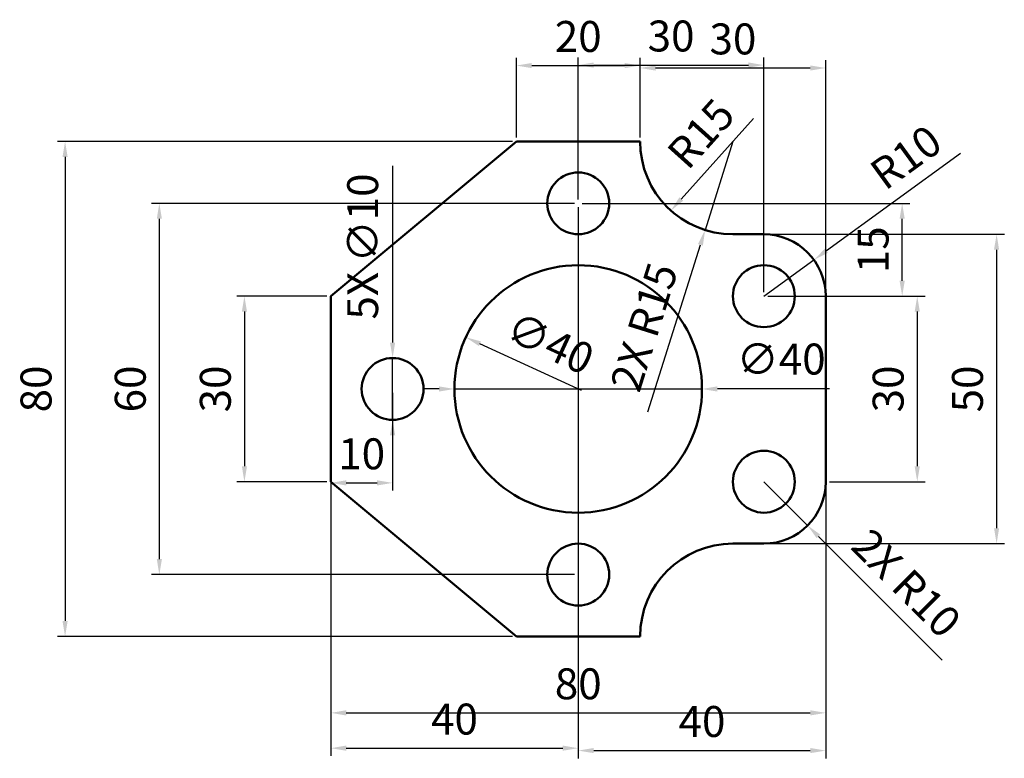
# Model space of a CAD drawing. Units: millimetres. Extents: x -90 to 69, y -60 to 60.
import ezdxf

# ---------------------------------------------------------------- set-up
doc = ezdxf.new("R2010")
doc.units = ezdxf.units.MM
doc.layers.add('M-DIMS', color=2, linetype='Continuous', lineweight=25)
doc.layers.add('M-OUTL', color=7, linetype='Continuous', lineweight=50)
doc.styles.get("Standard").update_dxf_attribs({"font": 'arial.ttf'})
doc.dimstyles.new('ISO-25', dxfattribs={"dimtxt": 5, "dimasz": 2.5, "dimexe": 1.25, "dimexo": 0.625, "dimgap": 1.5, "dimtad": 1, "dimdsep": 46, "dimtxsty": 'Standard', "dimcen": 4, "dimadec": 0, "dimazin": 0, "dimtfac": 1, "dimtmove": 0, "dimatfit": 3, "dimfxl": 1, "dimarcsym": 0})

# ---------------------------------------------------------------- blocks, each defined once
blk = doc.blocks.new('*D1')
at = {"layer": 'Defpoints', "color": 0, "transparency": 16777216}
for p in [(0, 30), (-40, -15), (0, -58.06)]:
    blk.add_point(p, dxfattribs=at)
at = {"layer": 'M-DIMS', "color": 0, "lineweight": -2, "transparency": 16777216}
for p, q in [((0, 29.38), (0, -59.31)), ((-40, -15.62), (-40, -59.31)), ((-37.5, -58.06), (-2.5, -58.06))]:
    blk.add_line(p, q, dxfattribs=at)
at = {"layer": 'M-DIMS', "color": 0, "transparency": 16777216}
for points in [[(-37.5, -57.64), (-37.5, -58.47), (-40, -58.06)], [(-2.5, -57.64), (-2.5, -58.47), (0, -58.06)]]:
    blk.add_solid(points, dxfattribs=at)
at = {"layer": 'M-DIMS', "color": 0, "transparency": 16777216, "insert": (-20, -54), "char_height": 5, "attachment_point": 5}
blk.add_mtext('40', dxfattribs=at)
blk = doc.blocks.new('*D2')
at = {"layer": 'Defpoints', "color": 0, "transparency": 16777216}
for p in [(40, -15), (0, -30), (40, -58.45)]:
    blk.add_point(p, dxfattribs=at)
at = {"layer": 'M-DIMS', "color": 0, "lineweight": -2, "transparency": 16777216}
for p, q in [((40, -15.62), (40, -59.7)), ((0, -30.62), (0, -59.7)), ((2.5, -58.45), (37.5, -58.45))]:
    blk.add_line(p, q, dxfattribs=at)
at = {"layer": 'M-DIMS', "color": 0, "transparency": 16777216}
for points in [[(2.5, -58.03), (2.5, -58.86), (0, -58.45)], [(37.5, -58.03), (37.5, -58.86), (40, -58.45)]]:
    blk.add_solid(points, dxfattribs=at)
at = {"layer": 'M-DIMS', "color": 0, "transparency": 16777216, "insert": (20, -54.39), "char_height": 5, "attachment_point": 5}
blk.add_mtext('40', dxfattribs=at)
blk = doc.blocks.new('*D3')
at = {"layer": 'Defpoints', "color": 0, "transparency": 16777216}
for p in [(-40, 15), (-53.95, -15), (-40, -15)]:
    blk.add_point(p, dxfattribs=at)
at = {"layer": 'M-DIMS', "color": 0, "lineweight": -2, "transparency": 16777216}
for p, q in [((-40.63, 15), (-55.2, 15)), ((-53.95, 12.5), (-53.95, -12.5)), ((-40.63, -15), (-55.2, -15))]:
    blk.add_line(p, q, dxfattribs=at)
at = {"layer": 'M-DIMS', "color": 0, "transparency": 16777216}
for points in [[(-54.36, 12.5), (-53.53, 12.5), (-53.95, 15)], [(-54.36, -12.5), (-53.53, -12.5), (-53.95, -15)]]:
    blk.add_solid(points, dxfattribs=at)
at = {"layer": 'M-DIMS', "color": 0, "transparency": 16777216, "insert": (-58, 0), "char_height": 5, "attachment_point": 5, "rotation": 90}
blk.add_mtext('30', dxfattribs=at)
blk = doc.blocks.new('*D4')
at = {"layer": 'Defpoints', "color": 0, "transparency": 16777216}
for p in [(0, 30), (-67.7, -30), (0, -30)]:
    blk.add_point(p, dxfattribs=at)
at = {"layer": 'M-DIMS', "color": 0, "lineweight": -2, "transparency": 16777216}
for p, q in [((-0.62, 30), (-68.95, 30)), ((-67.7, 27.5), (-67.7, -27.5)), ((-0.62, -30), (-68.95, -30))]:
    blk.add_line(p, q, dxfattribs=at)
at = {"layer": 'M-DIMS', "color": 0, "transparency": 16777216}
for points in [[(-68.11, 27.5), (-67.28, 27.5), (-67.7, 30)], [(-68.11, -27.5), (-67.28, -27.5), (-67.7, -30)]]:
    blk.add_solid(points, dxfattribs=at)
at = {"layer": 'M-DIMS', "color": 0, "transparency": 16777216, "insert": (-71.75, 0), "char_height": 5, "attachment_point": 5, "rotation": 90}
blk.add_mtext('60', dxfattribs=at)
blk = doc.blocks.new('*D5')
at = {"layer": 'Defpoints', "color": 0, "transparency": 16777216}
for p in [(-10, 40), (-82.93, -40), (-10, -40)]:
    blk.add_point(p, dxfattribs=at)
at = {"layer": 'M-DIMS', "color": 0, "lineweight": -2, "transparency": 16777216}
for p, q in [((-10.62, 40), (-84.18, 40)), ((-82.93, 37.5), (-82.93, -37.5)), ((-10.62, -40), (-84.18, -40))]:
    blk.add_line(p, q, dxfattribs=at)
at = {"layer": 'M-DIMS', "color": 0, "transparency": 16777216}
for points in [[(-83.35, 37.5), (-82.51, 37.5), (-82.93, 40)], [(-83.35, -37.5), (-82.51, -37.5), (-82.93, -40)]]:
    blk.add_solid(points, dxfattribs=at)
at = {"layer": 'M-DIMS', "color": 0, "transparency": 16777216, "insert": (-86.98, 0), "char_height": 5, "attachment_point": 5, "rotation": 90}
blk.add_mtext('80', dxfattribs=at)
blk = doc.blocks.new('*D6')
at = {"layer": 'Defpoints', "color": 0, "transparency": 16777216}
for p in [(10, 52.27), (-10, 40), (10, 40)]:
    blk.add_point(p, dxfattribs=at)
at = {"layer": 'M-DIMS', "color": 0, "lineweight": -2, "transparency": 16777216}
for p, q in [((-10, 40.62), (-10, 53.52)), ((10, 40.62), (10, 53.52)), ((-7.5, 52.27), (7.5, 52.27))]:
    blk.add_line(p, q, dxfattribs=at)
at = {"layer": 'M-DIMS', "color": 0, "transparency": 16777216}
for points in [[(-7.5, 52.69), (-7.5, 51.86), (-10, 52.27)], [(7.5, 52.69), (7.5, 51.86), (10, 52.27)]]:
    blk.add_solid(points, dxfattribs=at)
at = {"layer": 'M-DIMS', "color": 0, "transparency": 16777216, "insert": (0, 56.33), "char_height": 5, "attachment_point": 5}
blk.add_mtext('20', dxfattribs=at)
blk = doc.blocks.new('*D7')
at = {"layer": 'Defpoints', "color": 0, "transparency": 16777216}
for p in [(40, 51.88), (10, 40), (40, 15)]:
    blk.add_point(p, dxfattribs=at)
at = {"layer": 'M-DIMS', "color": 0, "lineweight": -2, "transparency": 16777216}
for p, q in [((10, 40.62), (10, 53.13)), ((40, 15.62), (40, 53.13)), ((12.5, 51.88), (37.5, 51.88))]:
    blk.add_line(p, q, dxfattribs=at)
at = {"layer": 'M-DIMS', "color": 0, "transparency": 16777216}
for points in [[(12.5, 52.29), (12.5, 51.46), (10, 51.88)], [(37.5, 52.29), (37.5, 51.46), (40, 51.88)]]:
    blk.add_solid(points, dxfattribs=at)
at = {"layer": 'M-DIMS', "color": 0, "transparency": 16777216, "insert": (25, 55.93), "char_height": 5, "attachment_point": 5}
blk.add_mtext('30', dxfattribs=at)
blk = doc.blocks.new('*D8')
at = {"layer": 'Defpoints', "color": 0, "transparency": 16777216}
for p in [(40, 15), (40, -15), (54.79, -15)]:
    blk.add_point(p, dxfattribs=at)
at = {"layer": 'M-DIMS', "color": 0, "lineweight": -2, "transparency": 16777216}
for p, q in [((40.63, 15), (56.04, 15)), ((54.79, 12.5), (54.79, -12.5)), ((40.63, -15), (56.04, -15))]:
    blk.add_line(p, q, dxfattribs=at)
at = {"layer": 'M-DIMS', "color": 0, "transparency": 16777216}
for points in [[(54.37, 12.5), (55.2, 12.5), (54.79, 15)], [(54.37, -12.5), (55.2, -12.5), (54.79, -15)]]:
    blk.add_solid(points, dxfattribs=at)
at = {"layer": 'M-DIMS', "color": 0, "transparency": 16777216, "insert": (50.73, 0), "char_height": 5, "attachment_point": 5, "rotation": 90}
blk.add_mtext('30', dxfattribs=at)
blk = doc.blocks.new('*D9')
at = {"layer": 'Defpoints', "color": 0, "transparency": 16777216}
for p in [(27.5, 25), (27.5, -25), (67.61, -25)]:
    blk.add_point(p, dxfattribs=at)
at = {"layer": 'M-DIMS', "color": 0, "lineweight": -2, "transparency": 16777216}
for p, q in [((28.13, 25), (68.86, 25)), ((67.61, 22.5), (67.61, -22.5)), ((28.13, -25), (68.86, -25))]:
    blk.add_line(p, q, dxfattribs=at)
at = {"layer": 'M-DIMS', "color": 0, "transparency": 16777216}
for points in [[(67.19, 22.5), (68.02, 22.5), (67.61, 25)], [(67.19, -22.5), (68.02, -22.5), (67.61, -25)]]:
    blk.add_solid(points, dxfattribs=at)
at = {"layer": 'M-DIMS', "color": 0, "transparency": 16777216, "insert": (63.55, 0), "char_height": 5, "attachment_point": 5, "rotation": 90}
blk.add_mtext('50', dxfattribs=at)
blk = doc.blocks.new('*D10')
at = {"layer": 'Defpoints', "color": 0, "transparency": 16777216}
for p in [(38.09, 20.87), (30, 15)]:
    blk.add_point(p, dxfattribs=at)
at = {"layer": 'M-DIMS', "color": 0, "lineweight": -2, "transparency": 16777216}
for p, q in [((61.76, 38.04), (40.12, 22.34)), ((30, 15), (38.09, 20.87))]:
    blk.add_line(p, q, dxfattribs=at)
at = {"layer": 'M-DIMS', "color": 0, "transparency": 16777216}
blk.add_solid([(39.87, 22.68), (40.36, 22), (38.09, 20.87)], dxfattribs=at)
at = {"layer": 'M-DIMS', "color": 0, "transparency": 16777216, "insert": (53.33, 36.94), "char_height": 5, "attachment_point": 5, "rotation": 35.9647}
blk.add_mtext('R10', dxfattribs=at)
blk = doc.blocks.new('*D11')
at = {"layer": 'Defpoints', "color": 0, "transparency": 16777216}
for p in [(25, 40), (14.98, 28.83)]:
    blk.add_point(p, dxfattribs=at)
at = {"layer": 'M-DIMS', "color": 0, "lineweight": -2, "transparency": 16777216}
blk.add_line((28.33, 43.71), (16.65, 30.7), dxfattribs=at)
at = {"layer": 'M-DIMS', "color": 0, "transparency": 16777216}
blk.add_solid([(16.34, 30.97), (16.96, 30.42), (14.98, 28.83)], dxfattribs=at)
at = {"layer": 'M-DIMS', "color": 0, "transparency": 16777216, "insert": (20.31, 40.84), "char_height": 5, "attachment_point": 5, "rotation": 48.1039}
blk.add_mtext('R15', dxfattribs=at)
blk = doc.blocks.new('*D12')
at = {"layer": 'Defpoints', "color": 0, "transparency": 16777216}
for p in [(-40, 0), (-30, 0), (-30, -15.18)]:
    blk.add_point(p, dxfattribs=at)
at = {"layer": 'M-DIMS', "color": 0, "lineweight": -2, "transparency": 16777216}
for p, q in [((-40, -0.62), (-40, -16.43)), ((-30, -0.62), (-30, -16.43)), ((-37.5, -15.18), (-32.5, -15.18))]:
    blk.add_line(p, q, dxfattribs=at)
at = {"layer": 'M-DIMS', "color": 0, "transparency": 16777216}
for points in [[(-37.5, -14.76), (-37.5, -15.6), (-40, -15.18)], [(-32.5, -14.76), (-32.5, -15.6), (-30, -15.18)]]:
    blk.add_solid(points, dxfattribs=at)
at = {"layer": 'M-DIMS', "color": 0, "transparency": 16777216, "insert": (-35, -11.13), "char_height": 5, "attachment_point": 5}
blk.add_mtext('10', dxfattribs=at)
blk = doc.blocks.new('*D13')
at = {"layer": 'Defpoints', "color": 0, "transparency": 16777216}
for p in [(-18.17, 8.36), (18.17, -8.36)]:
    blk.add_point(p, dxfattribs=at)
at = {"layer": 'M-DIMS', "color": 0, "lineweight": -2, "transparency": 16777216}
blk.add_line((0.53, -0.24), (-15.9, 7.31), dxfattribs=at)
at = {"layer": 'M-DIMS', "color": 0, "transparency": 16777216}
blk.add_solid([(-15.72, 7.69), (-16.07, 6.94), (-18.17, 8.36)], dxfattribs=at)
at = {"layer": 'M-DIMS', "color": 0, "transparency": 16777216, "insert": (-4.8, 6.82), "char_height": 5, "attachment_point": 5, "rotation": 335.2959}
blk.add_mtext('∅40', dxfattribs=at)
blk = doc.blocks.new('HOLE-D10')
blk.add_circle((5, 5), 5)
blk = doc.blocks.new('*D15')
at = {"layer": 'Defpoints', "color": 0, "transparency": 16777216}
for p in [(-40, -15), (40, -15), (40, -52.35)]:
    blk.add_point(p, dxfattribs=at)
at = {"layer": 'M-DIMS', "color": 0, "lineweight": -2, "transparency": 16777216}
for p, q in [((-40, -15.62), (-40, -53.6)), ((40, -15.62), (40, -53.6)), ((-37.5, -52.35), (37.5, -52.35))]:
    blk.add_line(p, q, dxfattribs=at)
at = {"layer": 'M-DIMS', "color": 0, "transparency": 16777216}
for points in [[(-37.5, -51.93), (-37.5, -52.77), (-40, -52.35)], [(37.5, -51.93), (37.5, -52.77), (40, -52.35)]]:
    blk.add_solid(points, dxfattribs=at)
at = {"layer": 'M-DIMS', "color": 0, "transparency": 16777216, "insert": (0, -48.3), "char_height": 5, "attachment_point": 5}
blk.add_mtext('80', dxfattribs=at)
blk = doc.blocks.new('*D16')
at = {"layer": 'Defpoints', "color": 0, "transparency": 16777216}
for p in [(30, 52.35), (0, 30), (30, 15)]:
    blk.add_point(p, dxfattribs=at)
at = {"layer": 'M-DIMS', "color": 0, "lineweight": -2, "transparency": 16777216}
for p, q in [((0, 30.62), (0, 53.6)), ((30, 15.62), (30, 53.6)), ((2.5, 52.35), (27.5, 52.35))]:
    blk.add_line(p, q, dxfattribs=at)
at = {"layer": 'M-DIMS', "color": 0, "transparency": 16777216}
for points in [[(2.5, 52.77), (2.5, 51.93), (0, 52.35)], [(27.5, 52.77), (27.5, 51.93), (30, 52.35)]]:
    blk.add_solid(points, dxfattribs=at)
at = {"layer": 'M-DIMS', "color": 0, "transparency": 16777216, "insert": (15, 56.4), "char_height": 5, "attachment_point": 5}
blk.add_mtext('30', dxfattribs=at)
blk = doc.blocks.new('*D17')
at = {"layer": 'Defpoints', "color": 0, "transparency": 16777216}
for p in [(0, 30), (52.35, 30), (30, 15)]:
    blk.add_point(p, dxfattribs=at)
at = {"layer": 'M-DIMS', "color": 0, "lineweight": -2, "transparency": 16777216}
for p, q in [((0.63, 30), (53.6, 30)), ((52.35, 17.5), (52.35, 27.5)), ((30.63, 15), (53.6, 15))]:
    blk.add_line(p, q, dxfattribs=at)
at = {"layer": 'M-DIMS', "color": 0, "transparency": 16777216}
for points in [[(51.93, 27.5), (52.77, 27.5), (52.35, 30)], [(51.93, 17.5), (52.77, 17.5), (52.35, 15)]]:
    blk.add_solid(points, dxfattribs=at)
at = {"layer": 'M-DIMS', "color": 0, "transparency": 16777216, "insert": (48.3, 22.5), "char_height": 5, "attachment_point": 5, "rotation": 90}
blk.add_mtext('15', dxfattribs=at)
blk = doc.blocks.new('*D18')
at = {"layer": 'Defpoints', "color": 0, "transparency": 16777216}
for p in [(-20, 0), (20, 0)]:
    blk.add_point(p, dxfattribs=at)
at = {"layer": 'M-DIMS', "color": 0, "lineweight": -2, "transparency": 16777216}
for p, q in [((-22.5, 0), (-25, 0)), ((-20, 0), (20, 0)), ((40.59, 0), (22.5, 0))]:
    blk.add_line(p, q, dxfattribs=at)
at = {"layer": 'M-DIMS', "color": 0, "transparency": 16777216}
for points in [[(-22.5, 0.42), (-22.5, -0.42), (-20, 0)], [(22.5, 0.42), (22.5, -0.42), (20, 0)]]:
    blk.add_solid(points, dxfattribs=at)
at = {"layer": 'M-DIMS', "color": 0, "transparency": 16777216, "insert": (32.79, 4.19), "char_height": 5, "attachment_point": 5}
blk.add_mtext('∅40', dxfattribs=at)
blk = doc.blocks.new('*D19')
at = {"layer": 'Defpoints', "color": 0, "transparency": 16777216}
for p in [(-30, 5), (-30, -5)]:
    blk.add_point(p, dxfattribs=at)
at = {"layer": 'M-DIMS', "color": 0, "lineweight": -2, "transparency": 16777216}
for p, q in [((-30, 36.06), (-30, 7.5)), ((-30, -5), (-30, 5)), ((-30, -7.5), (-30, -10))]:
    blk.add_line(p, q, dxfattribs=at)
at = {"layer": 'M-DIMS', "color": 0, "transparency": 16777216}
for points in [[(-30.42, 7.5), (-29.58, 7.5), (-30, 5)], [(-30.42, -7.5), (-29.58, -7.5), (-30, -5)]]:
    blk.add_solid(points, dxfattribs=at)
at = {"layer": 'M-DIMS', "color": 0, "transparency": 16777216, "insert": (-34.19, 23.03), "char_height": 5, "attachment_point": 5, "rotation": 90}
blk.add_mtext('5X ∅10', dxfattribs=at)
blk = doc.blocks.new('*D20')
at = {"layer": 'Defpoints', "color": 0, "transparency": 16777216}
for p in [(25, 40), (20.5, 25.69)]:
    blk.add_point(p, dxfattribs=at)
at = {"layer": 'M-DIMS', "color": 0, "lineweight": -2, "transparency": 16777216}
for p, q in [((25, 40), (20.5, 25.69)), ((11.26, -3.7), (19.75, 23.31))]:
    blk.add_line(p, q, dxfattribs=at)
at = {"layer": 'M-DIMS', "color": 0, "transparency": 16777216}
blk.add_solid([(19.35, 23.43), (20.15, 23.18), (20.5, 25.69)], dxfattribs=at)
at = {"layer": 'M-DIMS', "color": 0, "transparency": 16777216, "insert": (11.26, 9.82), "char_height": 5, "attachment_point": 5, "rotation": 72.5434}
blk.add_mtext('2X R15', dxfattribs=at)
blk = doc.blocks.new('*D21')
at = {"layer": 'Defpoints', "color": 0, "transparency": 16777216}
for p in [(30, -15), (37.07, -22.07)]:
    blk.add_point(p, dxfattribs=at)
at = {"layer": 'M-DIMS', "color": 0, "lineweight": -2, "transparency": 16777216}
for p, q in [((30, -15), (37.07, -22.07)), ((58.82, -43.82), (38.84, -23.84))]:
    blk.add_line(p, q, dxfattribs=at)
at = {"layer": 'M-DIMS', "color": 0, "transparency": 16777216}
blk.add_solid([(39.13, -23.54), (38.54, -24.13), (37.07, -22.07)], dxfattribs=at)
at = {"layer": 'M-DIMS', "color": 0, "transparency": 16777216, "insert": (52.58, -31.85), "char_height": 5, "attachment_point": 5, "rotation": 315}
blk.add_mtext('2X R10', dxfattribs=at)

msp = doc.modelspace()

# ---------------------------------------------------------------- linework, layer by layer
at = {"layer": 'M-OUTL'}
for p, q in [((-10, 40), (-40, 15)), ((0, 40), (-10, 40)), ((0, 40), (10, 40)), ((10, 40), (10, 40)), ((25, 25), (30, 25)), ((-40, 0), (-40, 15)), ((40, 15), (40, 0)), ((-40, 0), (-40, -15)), ((40, -15), (40, 0)), ((-10, -40), (-40, -15)), ((25, -25), (30, -25)), ((0, -40), (-10, -40)), ((0, -40), (10, -40)), ((10, -40), (10, -40))]:
    msp.add_line(p, q, dxfattribs=at)
msp.add_circle((0, 0), 20, dxfattribs=at)
for centre, radius, start, end in [((25, 40), 15, 180, 270), ((30, 15), 10, 0, 90), ((30, -15), 10, 270, 0), ((25, -40), 15, 90, 180)]:
    msp.add_arc(centre, radius, start, end, dxfattribs=at)

# ---------------------------------------------------------------- block references
for p in [(-5, 25), (25, 10), (-35, -5), (25, -20), (-5, -35)]:
    msp.add_blockref('HOLE-D10', p, dxfattribs=at)

# ---------------------------------------------------------------- dimensions: what is measured, and where the dimension line sits
at = {"layer": 'M-DIMS'}
for base, p1, p2, override, picture, middle in [((10, 52.275), (-10, 40), (10, 40), {"dimclrd": 0, "dimclre": 0, "dimclrt": 0}, '*D6', (0, 56.328)), ((30, 52.35), (0, 30), (30, 15), {"dimdec": 0, "dimlfac": 1, "dimrnd": 0, "dimzin": 0, "dimdsep": 46, "dimlunit": 2}, '*D16', (15, 56.405)), ((40, 51.878), (10, 40), (40, 15), {"dimclrd": 0, "dimclre": 0, "dimclrt": 0}, '*D7', (25, 55.932)), ((0, -58.055), (-40, -15), (0, 30), {"dimclrd": 0, "dimclre": 0, "dimclrt": 0}, '*D1', (-20, -54.003)), ((-30, -15.179), (-40, 0), (-30, 0), {"dimclrd": 0, "dimclre": 0, "dimclrt": 0}, '*D12', (-35, -11.126)), ((40, -52.35), (-40, -15), (40, -15), {"dimdec": 0, "dimlfac": 1, "dimrnd": 0, "dimzin": 0, "dimdsep": 46, "dimlunit": 2}, '*D15', (0, -48.297)), ((40, -58.446), (0, -30), (40, -15), {"dimclrd": 0, "dimclre": 0, "dimclrt": 0}, '*D2', (20, -54.393))]:
    dim = msp.add_linear_dim(base=base, p1=p1, p2=p2, dimstyle='ISO-25', override=override, dxfattribs=at)
    dim.commit()
    dim.dimension.update_dxf_attribs({"geometry": picture, "text_midpoint": middle})
for center, mpoint, picture, middle in [((25, 40), (14.983, 28.835), '*D11', (23.326, 38.134)), ((30, 15), (38.094, 20.873), '*D10', (55.714, 33.658))]:
    dim = msp.add_radius_dim(center=center, mpoint=mpoint, dimstyle='ISO-25', override={"dimclrd": 0, "dimclre": 0, "dimclrt": 0}, dxfattribs=at)
    dim.commit()
    dim.dimension.update_dxf_attribs({"geometry": picture, "text_midpoint": middle, "dimtype": 164})
for base, p1, p2, override, picture, middle in [((-82.931, -40), (-10, 40), (-10, -40), {"dimclrd": 0, "dimclre": 0, "dimclrt": 0}, '*D5', (-86.984, 0)), ((-67.696, -30), (0, 30), (0, -30), {"dimclrd": 0, "dimclre": 0, "dimclrt": 0}, '*D4', (-71.749, 0)), ((52.35, 30), (30, 15), (0, 30), {"dimdec": 0, "dimlfac": 1, "dimrnd": 0, "dimzin": 0, "dimdsep": 46, "dimlunit": 2}, '*D17', (48.297, 22.5)), ((67.605, -25), (27.5, 25), (27.5, -25), {"dimclrd": 0, "dimclre": 0, "dimclrt": 0}, '*D9', (63.552, 0)), ((-53.947, -15), (-40, 15), (-40, -15), {"dimclrd": 0, "dimclre": 0, "dimclrt": 0}, '*D3', (-58.001, 0)), ((54.785, -15), (40, 15), (40, -15), {"dimclrd": 0, "dimclre": 0, "dimclrt": 0}, '*D8', (50.731, 0))]:
    dim = msp.add_linear_dim(base=base, p1=p1, p2=p2, angle=90, dimstyle='ISO-25', override=override, dxfattribs=at)
    dim.commit()
    dim.dimension.update_dxf_attribs({"geometry": picture, "text_midpoint": middle})
for center, mpoint, picture, middle in [((25, 40), (20.5, 25.691), '*D20', (11.262, 9.824)), ((30, -15), (37.071, -22.071), '*D21', (52.58, -31.848))]:
    dim = msp.add_radius_dim(center=center, mpoint=mpoint, text='2X <>', dimstyle='ISO-25', override={"dimdec": 0, "dimlfac": 1, "dimrnd": 0, "dimzin": 0, "dimdsep": 46, "dimlunit": 2}, dxfattribs=at)
    dim.commit()
    dim.dimension.update_dxf_attribs({"geometry": picture, "text_midpoint": middle})
dim = msp.add_diameter_dim_2p(p1=(-30, -5), p2=(-30, 5), text='5X <>', dimstyle='ISO-25', override={"dimdec": 0, "dimlfac": 1, "dimrnd": 0, "dimzin": 0, "dimdsep": 46, "dimlunit": 2}, dxfattribs=at)
dim.commit()
dim.dimension.update_dxf_attribs({"geometry": '*D19', "text_midpoint": (-30, 23.031)})
for p1, p2, override, picture, middle in [((18.17, -8.359), (-18.17, 8.359), {"dimclrd": 0, "dimclre": 0, "dimclrt": 0}, '*D13', (-6.548, 3.012)), ((-20, 0), (20, 0), {"dimdec": 0, "dimlfac": 1, "dimrnd": 0, "dimzin": 0, "dimdsep": 46, "dimlunit": 2}, '*D18', (32.793, 0))]:
    dim = msp.add_diameter_dim_2p(p1=p1, p2=p2, dimstyle='ISO-25', override=override, dxfattribs=at)
    dim.commit()
    dim.dimension.update_dxf_attribs({"geometry": picture, "text_midpoint": middle, "dimtype": 163})

doc.saveas('drawing.dxf')
